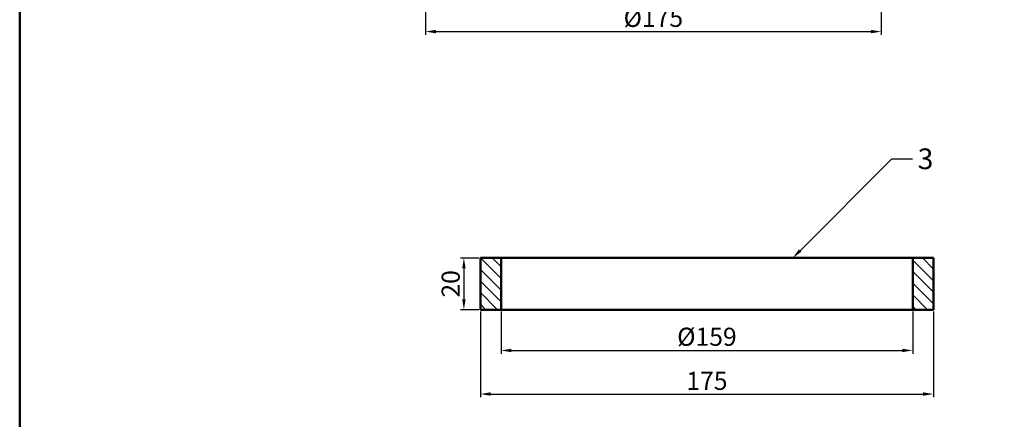
# Model space of a CAD drawing. Units: millimetres. Extents: x -21 to 693, y -570 to 295.
# Tile 2 of 7: x -21 to 359, y -159 to -4. Entities that reach past the tile are written whole.
import ezdxf
from ezdxf import colors
from ezdxf.entities.mleader import LeaderData, LeaderLine
from ezdxf.math import Vec2, Vec3

# ---------------------------------------------------------------- set-up
doc = ezdxf.new("R2010")
doc.units = ezdxf.units.MM
doc.header["$LTSCALE"] = 0.5
for name, color, linetype, lineweight in [('M-DIMS', 2, 'Continuous', 25), ('M-HATC', 8, 'Continuous', 18), ('M-OUTL', 7, 'Continuous', 50), ('M-TEXT', 3, 'Continuous', 25), ('M-TTLB', 7, 'Continuous', 50)]:
    doc.layers.add(name, color=color, linetype=linetype, lineweight=lineweight)
doc.styles.get("Standard").update_dxf_attribs({"font": 'arial.ttf'})
doc.dimstyles.new('ISO-25', dxfattribs={"dimtxt": 7, "dimasz": 4, "dimexe": 1.25, "dimexo": 0.625, "dimtad": 1, "dimdec": 0, "dimtxsty": 'Standard', "dimcen": 2.5, "dimadec": 0, "dimazin": 0, "dimtfac": 1, "dimtdec": 0, "dimtofl": 0, "dimtmove": 0, "dimatfit": 3, "dimfxl": 1, "dimarcsym": 0})

# ---------------------------------------------------------------- blocks, each defined once
blk = doc.blocks.new('*D5')
at = {"layer": 'Defpoints', "color": 0, "ltscale": 0.5, "transparency": 16777216}
for p in [(135.24, 81.11), (311.24, 81.11), (311.24, -8.97)]:
    blk.add_point(p, dxfattribs=at)
at = {"layer": 'M-DIMS', "color": 0, "lineweight": -2, "ltscale": 0.5, "transparency": 16777216}
for p, q in [((135.24, 80.49), (135.24, -10.22)), ((311.24, 80.49), (311.24, -10.22)), ((139.24, -8.97), (307.24, -8.97))]:
    blk.add_line(p, q, dxfattribs=at)
at = {"layer": 'M-DIMS', "color": 0, "ltscale": 0.5, "transparency": 16777216}
for points in [[(139.24, -8.31), (139.24, -9.64), (135.24, -8.97)], [(307.24, -8.31), (307.24, -9.64), (311.24, -8.97)]]:
    blk.add_solid(points, dxfattribs=at)
at = {"layer": 'M-DIMS', "color": 0, "ltscale": 0.5, "transparency": 16777216, "insert": (223.24, -4.58), "char_height": 7, "attachment_point": 5}
blk.add_mtext('%%C175', dxfattribs=at)
blk = doc.blocks.new('*D18')
at = {"layer": 'Defpoints', "color": 0, "ltscale": 0.5, "transparency": 16777216}
for p in [(156.43, -116.52), (331.43, -116.52), (331.43, -149.12)]:
    blk.add_point(p, dxfattribs=at)
at = {"layer": 'M-DIMS', "color": 0, "lineweight": -2, "ltscale": 0.5, "transparency": 16777216}
for p, q in [((156.43, -117.14), (156.43, -150.37)), ((331.43, -117.14), (331.43, -150.37)), ((160.43, -149.12), (327.43, -149.12))]:
    blk.add_line(p, q, dxfattribs=at)
at = {"layer": 'M-DIMS', "color": 0, "ltscale": 0.5, "transparency": 16777216}
for points in [[(160.43, -148.45), (160.43, -149.78), (156.43, -149.12)], [(327.43, -148.45), (327.43, -149.78), (331.43, -149.12)]]:
    blk.add_solid(points, dxfattribs=at)
at = {"layer": 'M-DIMS', "color": 0, "ltscale": 0.5, "transparency": 16777216, "insert": (243.93, -144.92), "char_height": 7, "attachment_point": 5}
blk.add_mtext('175', dxfattribs=at)
blk = doc.blocks.new('*D19')
at = {"layer": 'Defpoints', "color": 0, "ltscale": 0.5, "transparency": 16777216}
for p in [(164.43, -116.52), (323.43, -116.52), (323.43, -132.26)]:
    blk.add_point(p, dxfattribs=at)
at = {"layer": 'M-DIMS', "color": 0, "lineweight": -2, "ltscale": 0.5, "transparency": 16777216}
for p, q in [((164.43, -117.14), (164.43, -133.51)), ((323.43, -117.14), (323.43, -133.51)), ((168.43, -132.26), (319.43, -132.26))]:
    blk.add_line(p, q, dxfattribs=at)
at = {"layer": 'M-DIMS', "color": 0, "ltscale": 0.5, "transparency": 16777216}
for points in [[(168.43, -131.6), (168.43, -132.93), (164.43, -132.26)], [(319.43, -131.6), (319.43, -132.93), (323.43, -132.26)]]:
    blk.add_solid(points, dxfattribs=at)
at = {"layer": 'M-DIMS', "color": 0, "ltscale": 0.5, "transparency": 16777216, "insert": (243.93, -127.87), "char_height": 7, "attachment_point": 5}
blk.add_mtext('%%C159', dxfattribs=at)
blk = doc.blocks.new('*D20')
at = {"layer": 'Defpoints', "color": 0, "ltscale": 0.5, "transparency": 16777216}
for p in [(156.43, -96.52), (150.07, -116.52), (156.43, -116.52)]:
    blk.add_point(p, dxfattribs=at)
at = {"layer": 'M-DIMS', "color": 0, "lineweight": -2, "ltscale": 0.5, "transparency": 16777216}
for p, q in [((155.81, -96.52), (148.82, -96.52)), ((150.07, -100.52), (150.07, -112.52)), ((155.81, -116.52), (148.82, -116.52))]:
    blk.add_line(p, q, dxfattribs=at)
at = {"layer": 'M-DIMS', "color": 0, "ltscale": 0.5, "transparency": 16777216}
for points in [[(149.4, -100.52), (150.73, -100.52), (150.07, -96.52)], [(149.4, -112.52), (150.73, -112.52), (150.07, -116.52)]]:
    blk.add_solid(points, dxfattribs=at)
at = {"layer": 'M-DIMS', "color": 0, "ltscale": 0.5, "transparency": 16777216, "insert": (145.87, -106.52), "char_height": 7, "attachment_point": 5, "rotation": 90}
blk.add_mtext('20', dxfattribs=at)

msp = doc.modelspace()

# ---------------------------------------------------------------- hatches: boundary and pattern name
at = {"layer": 'M-HATC', "ltscale": 0.5}
h = msp.add_hatch(dxfattribs=at)
h.set_pattern_fill('ANSI31', color=256, angle=90)
h.set_pattern_definition([(135, (-182.564, -125.6284), (-2.245064, -2.245064), [])])
h.paths.add_polyline_path([(156.4318, -116.5165), (164.4318, -116.5165), (164.4318, -96.5165), (156.4318, -96.5165)])
h.paths.add_polyline_path([(323.4318, -116.5165), (331.4318, -116.5165), (331.4318, -96.5165), (323.4318, -96.5165)])

# ---------------------------------------------------------------- linework, layer by layer
at = {"layer": 'M-OUTL', "ltscale": 0.5}
for p, q in [((156.4318, -96.5165), (331.4318, -96.5165)), ((156.4318, -116.5165), (156.4318, -96.5165)), ((164.4318, -116.5165), (164.4318, -96.5165)), ((323.4318, -96.5165), (323.4318, -116.5165)), ((331.4318, -96.5165), (331.4318, -116.5165)), ((331.4318, -116.5165), (156.4318, -116.5165))]:
    msp.add_line(p, q, dxfattribs=at)
at = {"layer": 'M-TTLB', "ltscale": 0.5}
msp.add_lwpolyline([(-21.49, 295.4176), (693.1139, 295.4176), (693.1139, -570.0874), (-21.49, -570.0874)], close=True, dxfattribs=at)

# ---------------------------------------------------------------- dimensions: what is measured, and where the dimension line sits
at = {"layer": 'M-DIMS', "ltscale": 0.5}
dim = msp.add_linear_dim(base=(311.2368, -8.9735), p1=(135.2368, 81.1134), p2=(311.2368, 81.1134), text='%%C175', dimstyle='ISO-25', override={"dimclrd": 0, "dimclre": 0, "dimclrt": 0}, dxfattribs=at)
dim.commit()
dim.dimension.update_dxf_attribs({"geometry": '*D5', "text_midpoint": (223.2368, -8.9735), "dimtype": 160})
dim = msp.add_linear_dim(base=(150.0672, -116.5165), p1=(156.4318, -96.5165), p2=(156.4318, -116.5165), angle=90, dimstyle='ISO-25', override={"dimclrd": 0, "dimclre": 0, "dimclrt": 0}, dxfattribs=at)
dim.commit()
dim.dimension.update_dxf_attribs({"geometry": '*D20', "text_midpoint": (145.8682, -106.5165)})
dim = msp.add_linear_dim(base=(331.4318, -149.1165), p1=(156.4318, -116.5165), p2=(331.4318, -116.5165), dimstyle='ISO-25', override={"dimclrd": 0, "dimclre": 0, "dimclrt": 0}, dxfattribs=at)
dim.commit()
dim.dimension.update_dxf_attribs({"geometry": '*D18', "text_midpoint": (243.9318, -144.9175)})
dim = msp.add_linear_dim(base=(323.4318, -132.2627), p1=(164.4318, -116.5165), p2=(323.4318, -116.5165), text='%%C<>', dimstyle='ISO-25', override={"dimclrd": 0, "dimclre": 0, "dimclrt": 0}, dxfattribs=at)
dim.commit()
dim.dimension.update_dxf_attribs({"geometry": '*D19', "text_midpoint": (243.9318, -127.8679)})

# ---------------------------------------------------------------- leaders
at = {"layer": 'M-TEXT', "ltscale": 0.5}
ml = msp.add_multileader_mtext('Standard', dxfattribs=at)
ml.set_content('3', color=256)
ml.set_leader_properties()
ml.build(insert=Vec2(0, 0))
ctx = ml.context
ctx.base_point, ctx.char_height, ctx.plane_origin = Vec3(323.3429, -58.2383), 8, Vec3(277.0648, -96.5165)
notes = []
notes.append((ctx, [(0, (1, 1, 0), (315.3429, -58.2383), (1, 0), 8, [(0, [(277.0648, -96.5165)], 0, [])])]))
ctx.mtext.insert, ctx.mtext.flow_direction = Vec3(325.3429, -54.1674), 5
for ctx, leaders in notes:
    for number, flags, end, landing, length, lines in leaders:
        leader = LeaderData()
        leader.index, (leader.has_last_leader_line, leader.has_dogleg_vector, leader.attachment_direction) = number, flags
        leader.last_leader_point, leader.dogleg_vector, leader.dogleg_length = Vec3(end), Vec3(landing), length
        for number, points, colour, breaks in lines:
            line = LeaderLine()
            line.index, line.vertices, line.color, line.breaks = number, Vec3.list(points), colors.encode_raw_color(colour), breaks
            leader.lines.append(line)
        ctx.leaders.append(leader)

doc.saveas('drawing.dxf')
